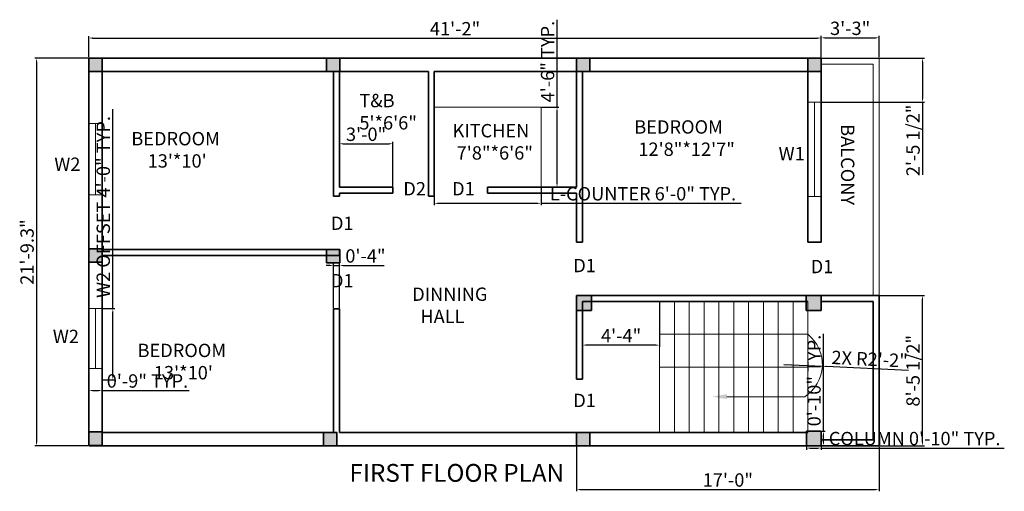
# Model space of a CAD drawing. Units: inches. Extents: x 107 to 1375, y 131 to 922.
# Tile 2 of 4: x 109 to 773, y 553 to 871. Entities that reach past the tile are written whole.
import ezdxf
from ezdxf import colors
from ezdxf.entities.mleader import LeaderData, LeaderLine
from ezdxf.math import Vec2, Vec3

# ---------------------------------------------------------------- set-up
doc = ezdxf.new("R2010")
doc.units = ezdxf.units.IN
for name, color, linetype, lineweight in [('A-ANNO-DIMS', 2, 'Continuous', 13), ('A-ANNO-TEXT', 7, 'Continuous', 18), ('A-ANNO-TITL', 7, 'Continuous', 25), ('A-AREA-IDEN', 7, 'Continuous', 18), ('A-COLS', 7, 'Continuous', 35), ('A-FLOR-FIXT', 8, 'Continuous', 18), ('A-FLOR-RAIL', 8, 'Continuous', 18), ('A-FLOR-STRS', 7, 'Continuous', 18), ('A-GLAZ', 4, 'Continuous', 18), ('A-WALL', 7, 'Continuous', 35)]:
    doc.layers.add(name, color=color, linetype=linetype, lineweight=lineweight)
doc.styles.get("Standard").update_dxf_attribs({"font": 'arial.ttf'})
doc.dimstyles.new('ISO-25', dxfattribs={"dimtxt": 9, "dimasz": 2.5, "dimexe": 1.25, "dimexo": 0.625, "dimtad": 1, "dimlunit": 3, "dimtxsty": 'Standard', "dimcen": 2.5, "dimadec": 0, "dimazin": 0, "dimtfac": 1, "dimtmove": 0, "dimatfit": 3, "dimfxl": 1, "dimarcsym": 0})

# ---------------------------------------------------------------- blocks, each defined once
blk = doc.blocks.new('*D3')
at = {"layer": 'A-ANNO-DIMS', "color": 0, "lineweight": -2, "transparency": 16777216}
for p, q in [((154.77, 845.33), (118.89, 845.33)), ((120.14, 842.83), (120.14, 586.53)), ((154.77, 584.03), (118.89, 584.03))]:
    blk.add_line(p, q, dxfattribs=at)
at = {"layer": 'A-ANNO-DIMS', "color": 0, "transparency": 16777216}
for points in [[(119.72, 842.83), (120.55, 842.83), (120.14, 845.33)], [(119.72, 586.53), (120.55, 586.53), (120.14, 584.03)]]:
    blk.add_solid(points, dxfattribs=at)
at = {"layer": 'Defpoints', "color": 0, "transparency": 16777216}
for p in [(155.4, 845.33), (120.14, 584.03), (155.4, 584.03)]:
    blk.add_point(p, dxfattribs=at)
at = {"layer": 'A-ANNO-DIMS', "color": 0, "transparency": 16777216, "insert": (114.91, 714.68), "char_height": 9, "attachment_point": 5, "rotation": 90}
blk.add_mtext('21\'-9.3"', dxfattribs=at)
blk = doc.blocks.new('*D4')
at = {"layer": 'A-ANNO-DIMS', "color": 0, "lineweight": -2, "transparency": 16777216}
for p, q in [((155.4, 845.96), (155.4, 860.19)), ((157.9, 858.94), (646.9, 858.94)), ((649.4, 845.96), (649.4, 860.19))]:
    blk.add_line(p, q, dxfattribs=at)
at = {"layer": 'A-ANNO-DIMS', "color": 0, "transparency": 16777216}
for points in [[(157.9, 859.35), (157.9, 858.52), (155.4, 858.94)], [(646.9, 859.35), (646.9, 858.52), (649.4, 858.94)]]:
    blk.add_solid(points, dxfattribs=at)
at = {"layer": 'Defpoints', "color": 0, "transparency": 16777216}
for p in [(649.4, 858.94), (155.4, 845.33), (649.4, 845.33)]:
    blk.add_point(p, dxfattribs=at)
at = {"layer": 'A-ANNO-DIMS', "color": 0, "transparency": 16777216, "insert": (402.4, 864.08), "char_height": 9, "attachment_point": 5}
blk.add_mtext('41\'-2"', dxfattribs=at)
blk = doc.blocks.new('*D5')
at = {"layer": 'A-ANNO-DIMS', "color": 0, "lineweight": -2, "transparency": 16777216}
for p, q in [((649.4, 845.96), (649.4, 860.35)), ((651.9, 859.1), (685.9, 859.1)), ((688.4, 845.96), (688.4, 860.35))]:
    blk.add_line(p, q, dxfattribs=at)
at = {"layer": 'A-ANNO-DIMS', "color": 0, "transparency": 16777216}
for points in [[(651.9, 859.51), (651.9, 858.68), (649.4, 859.1)], [(685.9, 859.51), (685.9, 858.68), (688.4, 859.1)]]:
    blk.add_solid(points, dxfattribs=at)
at = {"layer": 'Defpoints', "color": 0, "transparency": 16777216}
for p in [(688.4, 859.1), (649.4, 845.33), (688.4, 845.33)]:
    blk.add_point(p, dxfattribs=at)
at = {"layer": 'A-ANNO-DIMS', "color": 0, "transparency": 16777216, "insert": (668.9, 864.32), "char_height": 9, "attachment_point": 5}
blk.add_mtext('3\'-3"', dxfattribs=at)
blk = doc.blocks.new('COLUMN-10x10')
h = blk.add_hatch(color=256)
h.dxf.hatch_style = 1
h.paths.add_polyline_path([(10, 10), (0, 10), (0, 0), (10, 0)])
for p, q in [((10, 10), (0, 10)), ((0, 10), (0, 0)), ((10, 0), (10, 10)), ((0, 0), (10, 0))]:
    blk.add_line(p, q)
blk = doc.blocks.new('COLUMN-9x9')
h = blk.add_hatch(color=256)
h.dxf.hatch_style = 1
h.paths.add_polyline_path([(9, 9), (0, 9), (0, 0), (9, 0)])
blk.add_lwpolyline([(0, 0), (9, 0), (9, 9), (0, 9)], close=True)
blk = doc.blocks.new('WINDOW-PLAN-W1')
for p, q in [((0, 63.51), (0, 0)), ((0, 63.51), (9, 63.51)), ((4.5, 63.51), (4.5, 0)), ((9, 0), (9, 63.51)), ((0, 0), (9, 0))]:
    blk.add_line(p, q)
blk = doc.blocks.new('WINDOW-PLAN-W2-OFFSET')
for p, q in [((0, 48), (0, 0)), ((0, 48), (9, 48)), ((4.5, 48), (4.5, 7.53)), ((9, 0), (9, 48)), ((0, 7.53), (9, 7.53))]:
    blk.add_line(p, q)
blk = doc.blocks.new('WINDOW-PLAN-W2')
for p, q in [((0, 48), (0, 0)), ((0, 48), (9, 48)), ((4.5, 48), (4.5, 0)), ((9, 0), (9, 48)), ((0, 0), (9, 0))]:
    blk.add_line(p, q)
blk = doc.blocks.new('KITCHEN-COUNTER-L')
for q in [(0, 54), (72, 0)]:
    blk.add_line((72, 54), q)
blk = doc.blocks.new('*D22')
at = {"layer": 'A-ANNO-DIMS', "color": 0, "lineweight": -2, "transparency": 16777216}
for p, q in [((639.4, 583.41), (639.4, 581.28)), ((641.9, 582.53), (646.9, 582.53)), ((649.4, 583.41), (649.4, 581.28)), ((649.4, 582.53), (772.87, 582.53))]:
    blk.add_line(p, q, dxfattribs=at)
at = {"layer": 'A-ANNO-DIMS', "color": 0, "transparency": 16777216}
for points in [[(641.9, 582.95), (641.9, 582.11), (639.4, 582.53)], [(646.9, 582.95), (646.9, 582.11), (649.4, 582.53)]]:
    blk.add_solid(points, dxfattribs=at)
at = {"layer": 'Defpoints', "color": 0, "transparency": 16777216}
for p in [(639.4, 584.03), (649.4, 584.03), (649.4, 582.53)]:
    blk.add_point(p, dxfattribs=at)
at = {"layer": 'A-ANNO-DIMS', "color": 0, "transparency": 16777216, "insert": (712.38, 587.81), "char_height": 9, "attachment_point": 5}
blk.add_mtext('COLUMN 0\'-10" TYP.', dxfattribs=at)
blk = doc.blocks.new('*D23')
at = {"layer": 'A-ANNO-DIMS', "color": 0, "lineweight": -2, "transparency": 16777216}
for p, q in [((650.9, 594.03), (650.9, 659.63)), ((650.02, 594.03), (652.15, 594.03)), ((650.9, 586.53), (650.9, 591.53)), ((650.02, 584.03), (652.15, 584.03))]:
    blk.add_line(p, q, dxfattribs=at)
at = {"layer": 'A-ANNO-DIMS', "color": 0, "transparency": 16777216}
for points in [[(650.48, 591.53), (651.31, 591.53), (650.9, 594.03)], [(650.48, 586.53), (651.31, 586.53), (650.9, 584.03)]]:
    blk.add_solid(points, dxfattribs=at)
at = {"layer": 'Defpoints', "color": 0, "transparency": 16777216}
for p in [(649.4, 594.03), (650.9, 594.03), (649.4, 584.03)]:
    blk.add_point(p, dxfattribs=at)
at = {"layer": 'A-ANNO-DIMS', "color": 0, "transparency": 16777216, "insert": (645.68, 628.08), "char_height": 9, "attachment_point": 5, "rotation": 90}
blk.add_mtext('0\'-10" TYP.', dxfattribs=at)
blk = doc.blocks.new('*D26')
at = {"layer": 'A-ANNO-DIMS', "color": 0, "lineweight": -2, "transparency": 16777216}
for p, q in [((171.6, 676.6), (171.6, 811.02)), ((165.02, 676.6), (172.85, 676.6)), ((171.6, 631.1), (171.6, 674.1)), ((165.02, 628.6), (172.85, 628.6))]:
    blk.add_line(p, q, dxfattribs=at)
at = {"layer": 'A-ANNO-DIMS', "color": 0, "transparency": 16777216}
for points in [[(171.18, 674.1), (172.01, 674.1), (171.6, 676.6)], [(171.18, 631.1), (172.01, 631.1), (171.6, 628.6)]]:
    blk.add_solid(points, dxfattribs=at)
at = {"layer": 'Defpoints', "color": 0, "transparency": 16777216}
for p in [(164.4, 676.6), (171.6, 676.6), (164.4, 628.6)]:
    blk.add_point(p, dxfattribs=at)
at = {"layer": 'A-ANNO-DIMS', "color": 0, "transparency": 16777216, "insert": (166.32, 745.06), "char_height": 9, "attachment_point": 5, "rotation": 90}
blk.add_mtext('W2 OFFSET 4\'-0" TYP.', dxfattribs=at)
blk = doc.blocks.new('*D27')
at = {"layer": 'A-ANNO-DIMS', "color": 0, "lineweight": -2, "transparency": 16777216}
for p, q in [((155.4, 627.97), (155.4, 620.15)), ((164.4, 627.97), (164.4, 620.15)), ((157.9, 621.4), (161.9, 621.4)), ((164.4, 621.4), (223.01, 621.4))]:
    blk.add_line(p, q, dxfattribs=at)
at = {"layer": 'A-ANNO-DIMS', "color": 0, "transparency": 16777216}
for points in [[(157.9, 621.82), (157.9, 620.98), (155.4, 621.4)], [(161.9, 621.82), (161.9, 620.98), (164.4, 621.4)]]:
    blk.add_solid(points, dxfattribs=at)
at = {"layer": 'Defpoints', "color": 0, "transparency": 16777216}
for p in [(155.4, 628.6), (164.4, 628.6), (164.4, 621.4)]:
    blk.add_point(p, dxfattribs=at)
at = {"layer": 'A-ANNO-DIMS', "color": 0, "transparency": 16777216, "insert": (194.95, 626.62), "char_height": 9, "attachment_point": 5}
blk.add_mtext('0\'-9" TYP.', dxfattribs=at)
blk = doc.blocks.new('*D30')
at = {"layer": 'A-ANNO-DIMS', "color": 0, "lineweight": -2, "transparency": 16777216}
for p, q in [((388.4, 757.71), (388.4, 746.28)), ((460.4, 757.71), (460.4, 746.28)), ((390.9, 747.53), (457.9, 747.53)), ((460.4, 747.53), (595.44, 747.53))]:
    blk.add_line(p, q, dxfattribs=at)
at = {"layer": 'A-ANNO-DIMS', "color": 0, "transparency": 16777216}
for points in [[(390.9, 747.95), (390.9, 747.11), (388.4, 747.53)], [(457.9, 747.95), (457.9, 747.11), (460.4, 747.53)]]:
    blk.add_solid(points, dxfattribs=at)
at = {"layer": 'Defpoints', "color": 0, "transparency": 16777216}
for p in [(388.4, 758.33), (460.4, 758.33), (460.4, 747.53)]:
    blk.add_point(p, dxfattribs=at)
at = {"layer": 'A-ANNO-DIMS', "color": 0, "transparency": 16777216, "insert": (529.17, 752.81), "char_height": 9, "attachment_point": 5}
blk.add_mtext('L-COUNTER 6\'-0" TYP.', dxfattribs=at)
blk = doc.blocks.new('*D31')
at = {"layer": 'A-ANNO-DIMS', "color": 0, "lineweight": -2, "transparency": 16777216}
for p, q in [((471.2, 812.33), (471.2, 871.3)), ((461.02, 812.33), (472.45, 812.33)), ((471.2, 760.83), (471.2, 809.83)), ((461.02, 758.33), (472.45, 758.33))]:
    blk.add_line(p, q, dxfattribs=at)
at = {"layer": 'A-ANNO-DIMS', "color": 0, "transparency": 16777216}
for points in [[(470.78, 809.83), (471.61, 809.83), (471.2, 812.33)], [(470.78, 760.83), (471.61, 760.83), (471.2, 758.33)]]:
    blk.add_solid(points, dxfattribs=at)
at = {"layer": 'Defpoints', "color": 0, "transparency": 16777216}
for p in [(460.4, 812.33), (471.2, 812.33), (460.4, 758.33)]:
    blk.add_point(p, dxfattribs=at)
at = {"layer": 'A-ANNO-DIMS', "color": 0, "transparency": 16777216, "insert": (465.98, 843.07), "char_height": 9, "attachment_point": 5, "rotation": 90}
blk.add_mtext('4\'-6" TYP.', dxfattribs=at)
blk = doc.blocks.new('*D47')
at = {"layer": 'A-ANNO-DIMS', "color": 0, "lineweight": -2, "transparency": 16777216}
for p, q in [((324.4, 758.96), (324.4, 788.93)), ((326.9, 787.68), (357.9, 787.68)), ((360.4, 758.96), (360.4, 788.93))]:
    blk.add_line(p, q, dxfattribs=at)
at = {"layer": 'A-ANNO-DIMS', "color": 0, "transparency": 16777216}
for points in [[(326.9, 788.1), (326.9, 787.26), (324.4, 787.68)], [(357.9, 788.1), (357.9, 787.26), (360.4, 787.68)]]:
    blk.add_solid(points, dxfattribs=at)
at = {"layer": 'Defpoints', "color": 0, "transparency": 16777216}
for p in [(360.4, 787.68), (324.4, 758.33), (360.4, 758.33)]:
    blk.add_point(p, dxfattribs=at)
at = {"layer": 'A-ANNO-DIMS', "color": 0, "transparency": 16777216, "insert": (342.4, 792.9), "char_height": 9, "attachment_point": 5}
blk.add_mtext('3\'-0"', dxfattribs=at)
blk = doc.blocks.new('*D51')
at = {"layer": 'A-ANNO-DIMS', "color": 0, "lineweight": -2, "transparency": 16777216}
for p, q in [((650.02, 845.33), (719, 845.33)), ((717.75, 842.83), (717.75, 818.11)), ((650.02, 815.61), (719, 815.61)), ((717.75, 815.61), (717.75, 766.81))]:
    blk.add_line(p, q, dxfattribs=at)
at = {"layer": 'A-ANNO-DIMS', "color": 0, "transparency": 16777216}
for points in [[(717.33, 842.83), (718.16, 842.83), (717.75, 845.33)], [(717.33, 818.11), (718.16, 818.11), (717.75, 815.61)]]:
    blk.add_solid(points, dxfattribs=at)
at = {"layer": 'Defpoints', "color": 0, "transparency": 16777216}
for p in [(649.4, 845.33), (649.4, 815.61), (717.75, 815.61)]:
    blk.add_point(p, dxfattribs=at)
at = {"layer": 'A-ANNO-DIMS', "color": 0, "transparency": 16777216, "insert": (712.47, 789.96), "char_height": 9, "attachment_point": 5, "rotation": 90}
blk.add_mtext('2\'-5 1/2"', dxfattribs=at)
blk = doc.blocks.new('*D52')
at = {"layer": 'A-ANNO-DIMS', "color": 0, "lineweight": -2, "transparency": 16777216}
for p, q in [((689.02, 685.33), (719, 685.33)), ((717.75, 586.53), (717.75, 682.83)), ((689.02, 584.03), (719, 584.03))]:
    blk.add_line(p, q, dxfattribs=at)
at = {"layer": 'A-ANNO-DIMS', "color": 0, "transparency": 16777216}
for points in [[(717.33, 682.83), (718.16, 682.83), (717.75, 685.33)], [(717.33, 586.53), (718.16, 586.53), (717.75, 584.03)]]:
    blk.add_solid(points, dxfattribs=at)
at = {"layer": 'Defpoints', "color": 0, "transparency": 16777216}
for p in [(688.4, 685.33), (717.75, 685.33), (688.4, 584.03)]:
    blk.add_point(p, dxfattribs=at)
at = {"layer": 'A-ANNO-DIMS', "color": 0, "transparency": 16777216, "insert": (712.47, 634.68), "char_height": 9, "attachment_point": 5, "rotation": 90}
blk.add_mtext('8\'-5 1/2"', dxfattribs=at)
blk = doc.blocks.new('*D53')
at = {"layer": 'A-ANNO-DIMS', "color": 0, "lineweight": -2, "transparency": 16777216}
for p, q in [((484.4, 583.41), (484.4, 553.43)), ((688.4, 583.41), (688.4, 553.43)), ((486.9, 554.68), (685.9, 554.68))]:
    blk.add_line(p, q, dxfattribs=at)
at = {"layer": 'A-ANNO-DIMS', "color": 0, "transparency": 16777216}
for points in [[(486.9, 555.1), (486.9, 554.26), (484.4, 554.68)], [(685.9, 555.1), (685.9, 554.26), (688.4, 554.68)]]:
    blk.add_solid(points, dxfattribs=at)
at = {"layer": 'Defpoints', "color": 0, "transparency": 16777216}
for p in [(484.4, 584.03), (688.4, 584.03), (688.4, 554.68)]:
    blk.add_point(p, dxfattribs=at)
at = {"layer": 'A-ANNO-DIMS', "color": 0, "transparency": 16777216, "insert": (586.4, 559.9), "char_height": 9, "attachment_point": 5}
blk.add_mtext('17\'-0"', dxfattribs=at)
blk = doc.blocks.new('*D54')
at = {"layer": 'A-ANNO-DIMS', "color": 0, "lineweight": -2, "transparency": 16777216}
for p, q in [((488.4, 680.71), (488.4, 650.73)), ((540.4, 680.71), (540.4, 650.73)), ((537.9, 651.98), (490.9, 651.98))]:
    blk.add_line(p, q, dxfattribs=at)
at = {"layer": 'A-ANNO-DIMS', "color": 0, "transparency": 16777216}
for points in [[(490.9, 652.4), (490.9, 651.56), (488.4, 651.98)], [(537.9, 652.4), (537.9, 651.56), (540.4, 651.98)]]:
    blk.add_solid(points, dxfattribs=at)
at = {"layer": 'Defpoints', "color": 0, "transparency": 16777216}
for p in [(488.4, 681.33), (540.4, 681.33), (488.4, 651.98)]:
    blk.add_point(p, dxfattribs=at)
at = {"layer": 'A-ANNO-DIMS', "color": 0, "transparency": 16777216, "insert": (514.4, 657.11), "char_height": 9, "attachment_point": 5}
blk.add_mtext('4\'-4"', dxfattribs=at)
blk = doc.blocks.new('*D56')
at = {"layer": 'A-ANNO-DIMS', "color": 0, "lineweight": -2, "transparency": 16777216}
for p, q in [((317.9, 705.68), (315.4, 705.68)), ((320.4, 676.96), (320.4, 706.93)), ((320.4, 705.68), (324.4, 705.68)), ((324.4, 676.96), (324.4, 706.93)), ((326.9, 705.68), (354.57, 705.68))]:
    blk.add_line(p, q, dxfattribs=at)
at = {"layer": 'A-ANNO-DIMS', "color": 0, "transparency": 16777216}
for points in [[(317.9, 706.1), (317.9, 705.26), (320.4, 705.68)], [(326.9, 706.1), (326.9, 705.26), (324.4, 705.68)]]:
    blk.add_solid(points, dxfattribs=at)
at = {"layer": 'Defpoints', "color": 0, "transparency": 16777216}
for p in [(324.4, 705.68), (320.4, 676.33), (324.4, 676.33)]:
    blk.add_point(p, dxfattribs=at)
at = {"layer": 'A-ANNO-DIMS', "color": 0, "transparency": 16777216, "insert": (341.98, 710.9), "char_height": 9, "attachment_point": 5}
blk.add_mtext('0\'-4"', dxfattribs=at)
blk = doc.blocks.new('*D80')
at = {"layer": 'A-ANNO-DIMS', "color": 0, "lineweight": -2, "transparency": 16777216}
for p, q in [((624.18, 638.96), (650.14, 637.73)), ((708.35, 634.96), (652.63, 637.61))]:
    blk.add_line(p, q, dxfattribs=at)
at = {"layer": 'A-ANNO-DIMS', "color": 0, "transparency": 16777216}
blk.add_solid([(652.65, 638.03), (652.61, 637.19), (650.14, 637.73)], dxfattribs=at)
at = {"layer": 'Defpoints', "color": 0, "transparency": 16777216}
for p in [(624.18, 638.96), (650.14, 637.73)]:
    blk.add_point(p, dxfattribs=at)
at = {"layer": 'A-ANNO-DIMS', "color": 0, "transparency": 16777216, "insert": (681.99, 641.37), "char_height": 9, "attachment_point": 5, "rotation": 357.27704}
blk.add_mtext('2X R2\'-2"', dxfattribs=at)
blk = doc.blocks.new('STAIR-RETURN-PLAN')
for p, q in [((0, 0), (0, 88.3)), ((10, 0), (10, 88.3)), ((20, 0), (20, 88.3)), ((30, 0), (30, 88.3)), ((40, 0), (40, 88.3)), ((50, 0), (50, 88.3)), ((60, 0), (60, 88.3)), ((70, 0), (70, 88.3)), ((80, 0), (80, 88.3)), ((90, 0), (90, 88.3)), ((100, 0), (100, 88.3)), ((0, 66.24), (100, 66.24)), ((0, 44.15), (100, 44.15))]:
    blk.add_line(p, q)
for start, end in [(303.16419, 51.39065), (236.83581, 237.96095)]:
    blk.add_arc((83.79, 45.93), 25.99, start, end)
ml = blk.add_multileader_mtext('Standard')
ml.set_content('', color=256)
ml.set_leader_properties(color=256)
ml.build(insert=Vec2(0, 0))
ml.multileader.update_dxf_attribs({"arrow_head_size": 10})
ctx = ml.context
ctx.base_point, ctx.arrow_head_size, ctx.plane_origin = Vec3(98, 24.18), 10, Vec3(35.35, 24.18)
notes = []
notes.append((ctx, [(0, (1, 1, 0), (90, 24.18), (1, 0), 8, [(0, [(35.35, 24.18)], 0, [])])]))
ctx.mtext.insert, ctx.mtext.flow_direction = Vec3(100, 26.18), 5
for ctx, leaders in notes:
    for number, flags, end, landing, length, lines in leaders:
        leader = LeaderData()
        leader.index, (leader.has_last_leader_line, leader.has_dogleg_vector, leader.attachment_direction) = number, flags
        leader.last_leader_point, leader.dogleg_vector, leader.dogleg_length = Vec3(end), Vec3(landing), length
        for number, points, colour, breaks in lines:
            line = LeaderLine()
            line.index, line.vertices, line.color, line.breaks = number, Vec3.list(points), colors.encode_raw_color(colour), breaks
            leader.lines.append(line)
        ctx.leaders.append(leader)

msp = doc.modelspace()

# ---------------------------------------------------------------- linework, layer by layer
at = {"layer": 'A-FLOR-RAIL'}
for p, q in [((688.397, 845.331), (649.397, 845.331)), ((688.397, 685.331), (688.397, 845.331)), ((684.397, 841.331), (649.397, 841.331)), ((684.397, 685.331), (684.397, 841.331))]:
    msp.add_line(p, q, dxfattribs=at)
at = {"layer": 'A-WALL'}
for p, q in [((649.397, 845.331), (155.397, 845.331)), ((155.397, 845.331), (155.397, 584.031)), ((649.397, 721.331), (649.397, 845.331)), ((320.397, 836.331), (164.397, 836.331)), ((164.397, 836.331), (164.397, 716.331)), ((320.397, 836.331), (320.397, 752.331)), ((384.397, 836.331), (324.397, 836.331)), ((324.397, 836.331), (324.397, 758.331)), ((384.397, 836.331), (384.397, 752.331)), ((484.397, 836.331), (388.397, 836.331)), ((402.397, 836.331), (388.397, 836.331)), ((388.397, 836.331), (388.397, 752.331)), ((484.397, 836.331), (484.397, 758.331)), ((640.397, 836.331), (488.397, 836.331)), ((488.397, 836.331), (488.397, 721.331)), ((640.397, 721.331), (640.397, 836.331)), ((360.397, 758.331), (324.397, 758.331)), ((360.397, 758.331), (360.397, 754.331)), ((484.397, 758.331), (424.397, 758.331)), ((424.397, 758.331), (424.397, 754.331)), ((320.397, 752.331), (324.397, 752.331)), ((360.397, 754.331), (324.397, 754.331)), ((324.397, 754.331), (324.397, 752.331)), ((384.397, 752.331), (388.397, 752.331)), ((484.397, 754.331), (424.397, 754.331)), ((484.397, 754.331), (484.397, 721.331)), ((488.397, 721.331), (484.397, 721.331)), ((640.397, 721.331), (649.397, 721.331)), ((324.397, 716.331), (164.397, 716.331)), ((324.397, 712.331), (164.397, 712.331)), ((164.397, 712.331), (164.397, 593.031)), ((324.397, 716.331), (324.397, 712.331)), ((640.397, 685.331), (484.397, 685.331)), ((484.397, 685.331), (484.397, 629.031)), ((640.397, 685.331), (688.397, 685.331)), ((649.319, 685.331), (649.319, 681.331)), ((688.397, 685.331), (688.397, 584.031)), ((640.397, 681.331), (488.397, 681.331)), ((488.397, 681.331), (488.397, 629.031)), ((649.319, 681.331), (684.397, 681.331)), ((684.397, 681.331), (684.397, 588.031)), ((320.397, 676.331), (320.397, 593.031)), ((324.397, 676.331), (320.397, 676.331)), ((324.397, 676.331), (324.397, 593.031)), ((484.397, 629.031), (488.397, 629.031)), ((164.397, 593.031), (320.397, 593.031)), ((324.397, 593.031), (640.397, 593.031)), ((684.397, 588.031), (649.397, 588.031)), ((649.397, 588.031), (649.397, 584.031)), ((155.397, 584.031), (649.397, 584.031)), ((688.397, 584.031), (649.397, 584.031))]:
    msp.add_line(p, q, dxfattribs=at)

# ---------------------------------------------------------------- block references
at = {"layer": 'A-COLS'}
for name, p in [('COLUMN-9x9', (155.397, 836.331)), ('COLUMN-9x9', (315.721, 836.331)), ('COLUMN-9x9', (484.336, 836.331)), ('COLUMN-9x9', (640.354, 836.331)), ('COLUMN-9x9', (155.397, 707.82)), ('COLUMN-9x9', (315.659, 707.331)), ('COLUMN-10x10', (484.397, 675.331)), ('COLUMN-10x10', (639.319, 675.331)), ('COLUMN-9x9', (155.397, 584.405)), ('COLUMN-9x9', (313.71, 584.031)), ('COLUMN-9x9', (484.397, 584.031)), ('COLUMN-10x10', (639.397, 584.031))]:
    msp.add_blockref(name, p, dxfattribs=at)
at = {"layer": 'A-FLOR-FIXT'}
msp.add_blockref('KITCHEN-COUNTER-L', (388.397, 758.331), dxfattribs=at)
at = {"layer": 'A-FLOR-STRS'}
msp.add_blockref('STAIR-RETURN-PLAN', (540.397, 593.031), dxfattribs=at)
at = {"layer": 'A-GLAZ'}
for name, p in [('WINDOW-PLAN-W1', (640.397, 752.102)), ('WINDOW-PLAN-W2', (155.397, 753.304)), ('WINDOW-PLAN-W2-OFFSET', (155.397, 628.599))]:
    msp.add_blockref(name, p, dxfattribs=at)

# ---------------------------------------------------------------- texts
at = {"layer": 'A-ANNO-TEXT', "char_height": 9, "attachment_point": 1}
for s, insert in [('W1', (620.644, 785.454)), ('W2', (132.141, 778.375)), ('D2', (367.525, 761.857)), ('D1', (400.427, 761.857)), ('D1', (318.726, 738.617)), ('D1', (482.182, 710.105)), ('D1', (642.301, 709.434)), ('D1', (318.726, 699.877)), ('W2', (131.147, 662.311)), ('D1', (482.182, 619.183))]:
    msp.add_mtext_dynamic_manual_height_columns(s, width=33.2577, gutter_width=12.5, heights=[0], dxfattribs=dict(at, insert=insert))
at = {"layer": 'A-ANNO-TITL', "insert": (331.201, 571.838), "char_height": 12, "attachment_point": 1}
msp.add_mtext_dynamic_manual_height_columns('FIRST FLOOR PLAN', width=244.216, gutter_width=12.5, heights=[0], dxfattribs=at)
at = {"layer": 'A-AREA-IDEN', "char_height": 9, "attachment_point": 1}
for s, width, insert in [('T&B\\P5\'*6\'6"', 26.62767, (337.879, 821.301)), ('BEDROOM\\P 12\'8"*12\'7"', 89.49012, (523.321, 803.508)), ('KITCHEN\\P 7\'8"*6\'6"', 54.9024, (400.742, 801.004)), ("BEDROOM\\P    13'*10'", 64.41797, (184.073, 795.609)), ('DINNING\\P  HALL ', 53.67099, (373.54, 690.777)), ("BEDROOM\\P    13'*10'", 64.41797, (188.274, 652.883))]:
    msp.add_mtext_dynamic_manual_height_columns(s, width=width, gutter_width=12.5, heights=[0], dxfattribs=dict(at, insert=insert))
at = {"layer": 'A-AREA-IDEN', "insert": (671.725, 800.896), "char_height": 9, "attachment_point": 1, "rotation": 270}
msp.add_mtext_dynamic_manual_height_columns('BALCONY', width=55.17107, gutter_width=12.5, heights=[0], dxfattribs=at)

# ---------------------------------------------------------------- dimensions: what is measured, and where the dimension line sits
at = {"layer": 'A-ANNO-DIMS'}
for base, p1, p2, override, picture, middle in [((649.397, 858.935), (155.397, 845.331), (649.397, 845.331), {"dimclrd": 0, "dimclre": 0, "dimclrt": 0}, '*D4', (402.397, 864.079)), ((688.397, 859.097), (649.397, 845.331), (688.397, 845.331), {"dimclrd": 0, "dimclre": 0, "dimclrt": 0}, '*D5', (668.897, 864.32)), ((360.397, 787.681), (324.397, 758.331), (360.397, 758.331), {"dimdec": 1, "dimlfac": 1, "dimrnd": 0, "dimzin": 1, "dimdsep": 46, "dimlunit": 4, "dimfrac": 2}, '*D47', (342.397, 792.905)), ((324.397, 705.681), (320.397, 676.331), (324.397, 676.331), {"dimdec": 1, "dimlfac": 1, "dimrnd": 0, "dimzin": 1, "dimdsep": 46, "dimlunit": 4, "dimfrac": 2}, '*D56', (341.984, 710.902)), ((688.397, 554.681), (484.397, 584.031), (688.397, 584.031), {"dimdec": 1, "dimlfac": 1, "dimrnd": 0, "dimzin": 1, "dimdsep": 46, "dimlunit": 4, "dimfrac": 2}, '*D53', (586.397, 559.902))]:
    dim = msp.add_linear_dim(base=base, p1=p1, p2=p2, dimstyle='ISO-25', override=override, dxfattribs=at)
    dim.commit()
    dim.dimension.update_dxf_attribs({"geometry": picture, "text_midpoint": middle})
for base, p1, p2, text, picture, middle in [((471.197, 812.331), (460.397, 758.331), (460.397, 812.331), '<> TYP.', '*D31', (465.977, 843.067)), ((171.597, 676.599), (164.397, 628.599), (164.397, 676.599), 'W2 OFFSET <> TYP.', '*D26', (166.315, 745.057)), ((650.897, 594.031), (649.397, 584.031), (649.397, 594.031), '<> TYP.', '*D23', (645.677, 628.082))]:
    dim = msp.add_linear_dim(base=base, p1=p1, p2=p2, angle=90, text=text, dimstyle='ISO-25', override={"dimdec": 1, "dimlfac": 1, "dimrnd": 0, "dimzin": 1, "dimdsep": 46, "dimlunit": 4, "dimfrac": 2}, dxfattribs=at)
    dim.commit()
    dim.dimension.update_dxf_attribs({"geometry": picture, "text_midpoint": middle})
for base, p1, p2, angle, override, picture, middle in [((120.135, 584.031), (155.397, 845.331), (155.397, 584.031), 90, {"dimclrd": 0, "dimclre": 0, "dimclrt": 0}, '*D3', (114.912, 714.681)), ((717.747, 815.61), (649.397, 845.331), (649.397, 815.61), 90, {"dimdec": 1, "dimlfac": 1, "dimrnd": 0, "dimzin": 1, "dimdsep": 46, "dimlunit": 4, "dimfrac": 2}, '*D51', (712.468, 789.961)), ((717.747, 685.331), (688.397, 584.031), (688.397, 685.331), 90, {"dimdec": 1, "dimlfac": 1, "dimrnd": 0, "dimzin": 1, "dimdsep": 46, "dimlunit": 4, "dimfrac": 2}, '*D52', (712.468, 634.681)), ((488.397, 651.981), (540.397, 681.331), (488.397, 681.331), 180, {"dimdec": 1, "dimlfac": 1, "dimrnd": 0, "dimzin": 1, "dimdsep": 46, "dimlunit": 4, "dimfrac": 2}, '*D54', (514.397, 657.106))]:
    dim = msp.add_linear_dim(base=base, p1=p1, p2=p2, angle=angle, dimstyle='ISO-25', override=override, dxfattribs=at)
    dim.commit()
    dim.dimension.update_dxf_attribs({"geometry": picture, "text_midpoint": middle})
for base, p1, p2, text, picture, middle in [((460.397, 747.531), (388.397, 758.331), (460.397, 758.331), 'L-COUNTER <> TYP.', '*D30', (529.171, 752.813)), ((164.397, 621.399), (155.397, 628.599), (164.397, 628.599), '<> TYP.', '*D27', (194.951, 626.62)), ((649.397, 582.531), (639.397, 584.031), (649.397, 584.031), 'COLUMN <> TYP.', '*D22', (712.385, 587.813))]:
    dim = msp.add_linear_dim(base=base, p1=p1, p2=p2, text=text, dimstyle='ISO-25', override={"dimdec": 1, "dimlfac": 1, "dimrnd": 0, "dimzin": 1, "dimdsep": 46, "dimlunit": 4, "dimfrac": 2}, dxfattribs=at)
    dim.commit()
    dim.dimension.update_dxf_attribs({"geometry": picture, "text_midpoint": middle})
dim = msp.add_radius_dim(center=(624.182, 638.962), mpoint=(650.138, 637.728), text='2X <>', dimstyle='ISO-25', override={"dimdec": 1, "dimlfac": 1, "dimrnd": 0, "dimzin": 1, "dimdsep": 46, "dimlunit": 4, "dimfrac": 2}, dxfattribs=at)
dim.commit()
dim.dimension.update_dxf_attribs({"geometry": '*D80', "text_midpoint": (681.986, 641.366)})

doc.saveas('drawing.dxf')
